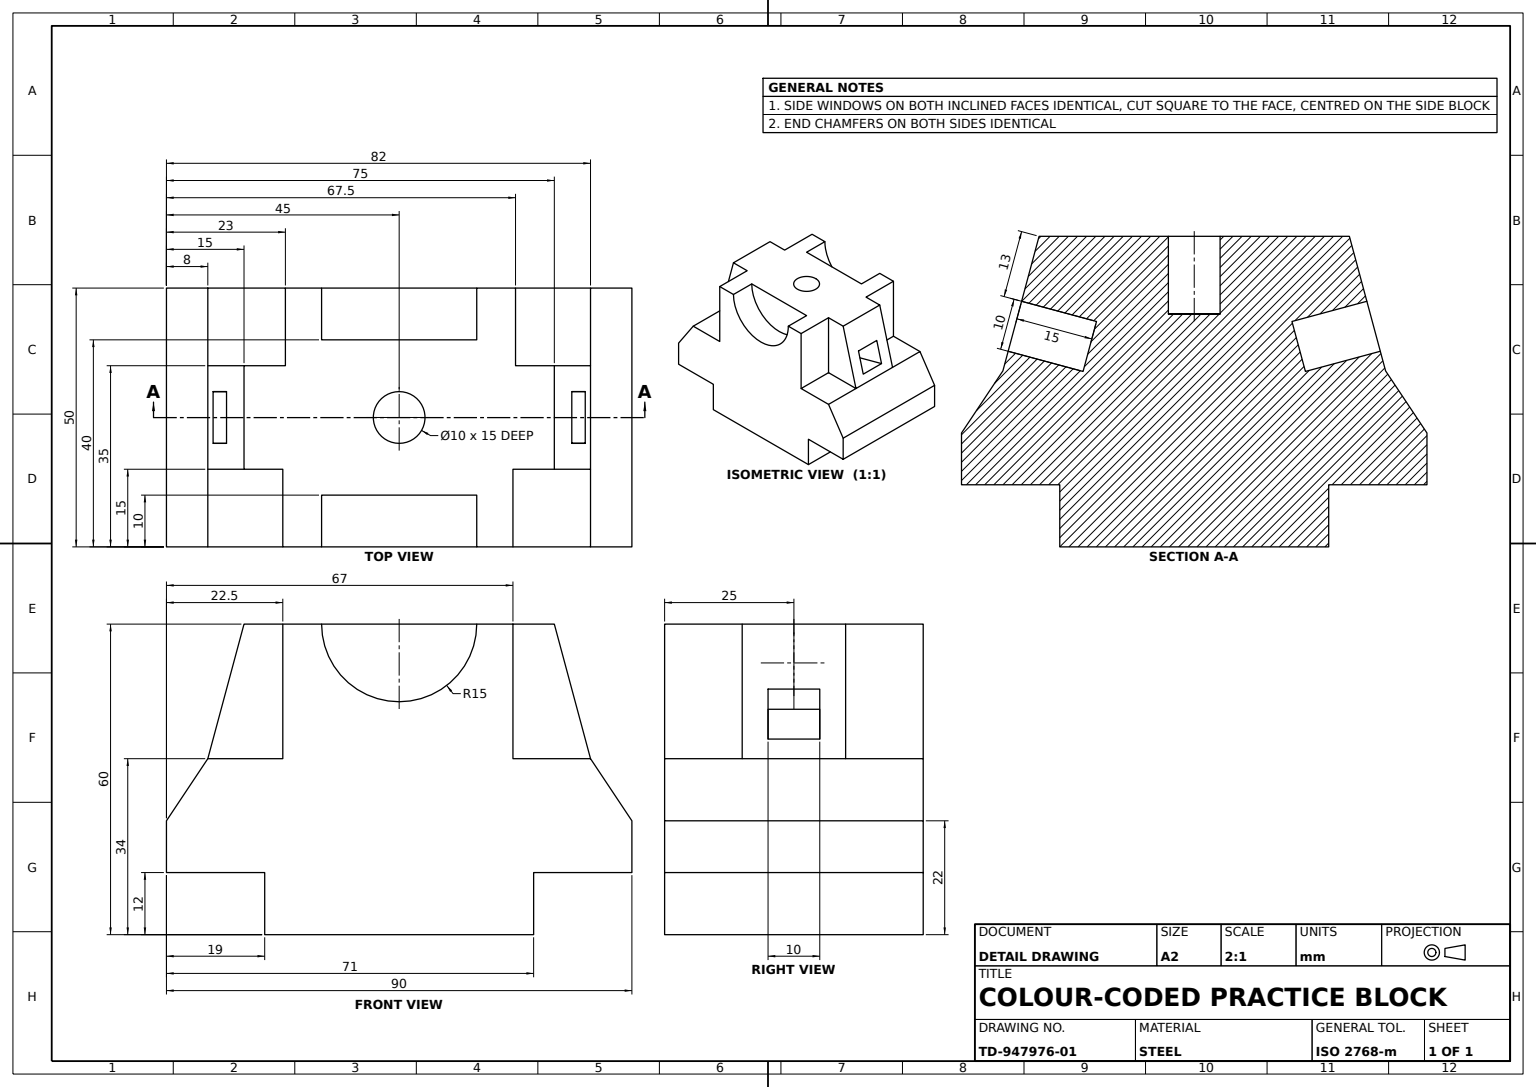
from build123d import *

# Parameters (mm, degrees)
BASE_BLOCK_DEPTH        = 50
SADDLE_CUT_1_30_DEPTH   = 10
SADDLE_START            = -10
SADDLE_CUT_2_30_DEPTH   = 10
UPPER_BLOCK_DEPTH       = 30
UPPER_BLOCK_NOTCH_DEPTH = 20
NOTCH_PAD_1_DEPTH       = 5
NOTCH_PAD_2_DEPTH       = 5
SIDE_BLOCK_DEPTH        = 35
SIDE_BLOCK_POCKET_DEPTH = 15
TOP_HOLE_SKETCH_R       = 5
TOP_HOLE_10_DEPTH       = 15
SIDE_WINDOW_SKETCH_W    = 10
SIDE_WINDOW_SKETCH_H    = 10
SIDE_WINDOW_CUT_DEPTH   = 15
UPPER_WINDOW_SKETCH_W   = 10
UPPER_WINDOW_SKETCH_H   = 10
UPPER_WINDOW_CUT_DEPTH  = 15


with BuildPart() as part:
    # Base Profile Sketch → Base Block (new body)
    with BuildSketch(Plane.XY):
        Polygon((0, 0), (52, 0), (52, 12), (71, 12), (71, 22), (63, 34), (48, 34), (48, 60), (4, 60), (4, 34), (-11, 34), (-19, 22), (-19, 12), (0, 12), align=None)
    extrude(amount=BASE_BLOCK_DEPTH)

    # Saddle Cut 1 Sketch → Saddle Cut 1 Ø30 (cut)
    with BuildSketch(Plane.XY.offset(50)):
        with BuildLine():
            Line((11, 60), (41, 60))
            ThreePointArc((41, 60), (26, 45), (11, 60))
        make_face()
    extrude(amount=-SADDLE_CUT_1_30_DEPTH, mode=Mode.SUBTRACT)

    # Saddle Cut 2 Sketch → Saddle Cut 2 Ø30 (cut)
    with BuildSketch(Plane(origin=(0, 0, 0), x_dir=(-1, 0, 0), z_dir=(0, 0, -1)).offset(SADDLE_START)):
        with BuildLine():
            Line((-41, 60), (-11, 60))
            ThreePointArc((-11, 60), (-26, 45), (-41, 60))
        make_face()
    extrude(amount=SADDLE_CUT_2_30_DEPTH, mode=Mode.SUBTRACT)

    # Upper Block Sketch → Upper Block (add)
    with BuildSketch(Plane(origin=(0, 0, 0), x_dir=(-1, 0, 0), z_dir=(0, 0, -1))):
        Polygon((-48, 60), (-48, 34), (-63, 34), (-56, 60), align=None)
    extrude(amount=-UPPER_BLOCK_DEPTH)

    # Upper Block Notch Sketch → Upper Block Notch (cut)
    with BuildSketch(Plane(origin=(0, 0, 0), x_dir=(-1, 0, 0), z_dir=(0, 0, -1))):
        Polygon((-63, 34), (-56, 60), (-48.5, 60), (-48.5, 34), align=None)
    extrude(amount=-UPPER_BLOCK_NOTCH_DEPTH, mode=Mode.SUBTRACT)

    # Notch Pad 1 Sketch → Notch Pad 1 (add)
    with BuildSketch(Plane(origin=(0, 0, 20), x_dir=(-1, 0, 0), z_dir=(0, 0, -1))):
        Polygon((-63, 34), (-48.5, 34), (-48.5, 60), (-56, 60), align=None)
    extrude(amount=NOTCH_PAD_1_DEPTH)

    # Notch Pad 2 Sketch → Notch Pad 2 (add)
    with BuildSketch(Plane.XY.offset(30)):
        Polygon((48, 60), (56, 60), (63, 34), (48, 34), align=None)
    extrude(amount=NOTCH_PAD_2_DEPTH)

    # Side Block Sketch → Side Block (add)
    with BuildSketch(Plane.XY.offset(50)):
        Polygon((4, 60), (4, 34), (-11, 34), (-4, 60), align=None)
    extrude(amount=-SIDE_BLOCK_DEPTH)

    # Side Block Pocket Sketch → Side Block Pocket (cut)
    with BuildSketch(Plane.XY.offset(50)):
        Polygon((3.5, 60), (3.5, 34), (-11, 34), (-4, 60), align=None)
    extrude(amount=-SIDE_BLOCK_POCKET_DEPTH, mode=Mode.SUBTRACT)

    # Top Hole Sketch → Top Hole Ø10 (cut)
    with BuildSketch(Plane(origin=(0, 60, 0), x_dir=(1, 0, 0), z_dir=(0, 1, 0))):
        with Locations(Location((26, -25, 0), (0, 0, 270))):
            Circle(TOP_HOLE_SKETCH_R)
    extrude(amount=-TOP_HOLE_10_DEPTH, mode=Mode.SUBTRACT)

    # Side Window Sketch → Side Window Cut (cut)
    with BuildSketch(Plane(origin=(-18.791724138, 5.059310345, 0), x_dir=(0, 0, 1), z_dir=(-0.9656157585206698, 0.25997347344787275, 0))):
        with Locations((25, 38.897051617)):
            Rectangle(SIDE_WINDOW_SKETCH_W, SIDE_WINDOW_SKETCH_H)
    extrude(amount=-SIDE_WINDOW_CUT_DEPTH, mode=Mode.SUBTRACT)

    # Upper Window Sketch → Upper Window Cut (cut)
    with BuildSketch(Plane(origin=(67.277241379, 18.113103448, 0), x_dir=(0, 0, -1), z_dir=(0.9656157585206697, 0.2599734734478728, 0))):
        with Locations((-25, 25.378430998)):
            Rectangle(UPPER_WINDOW_SKETCH_W, UPPER_WINDOW_SKETCH_H)
    extrude(amount=-UPPER_WINDOW_CUT_DEPTH, mode=Mode.SUBTRACT)


solid = part.part
